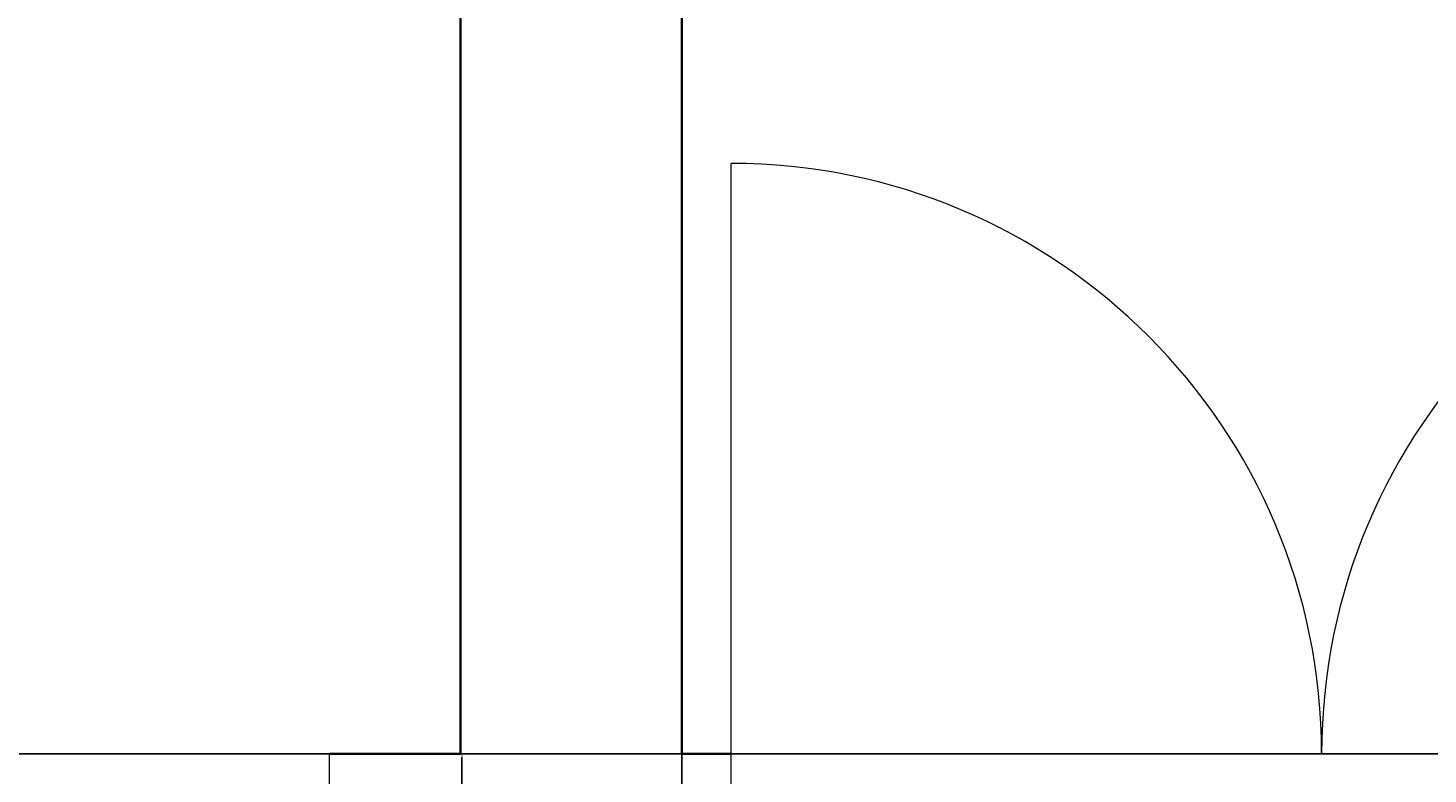
# Model space of a CAD drawing. Units: feet. Extents: x 1654 to 2985, y 1348 to 2230.
# Tile 32 of 53: x 2044 to 2100, y 1750 to 1781. Entities that reach past the tile are written whole.
import ezdxf

# ---------------------------------------------------------------- set-up
doc = ezdxf.new("R2010")
doc.units = ezdxf.units.FT
for name, color, linetype, lineweight in [('A-ANNO-DIMS', 2, 'Continuous', 18), ('A-DOOR', 3, 'Continuous', 18), ('A-WALL', 7, 'Continuous', 35), ('A-WALL-OPEN', 4, 'Continuous', 18)]:
    doc.layers.add(name, color=color, linetype=linetype, lineweight=lineweight)
doc.styles.get("Standard").update_dxf_attribs({"font": 'arial.ttf'})
doc.dimstyles.get("Standard").update_dxf_attribs({"dimtxt": 0.18, "dimasz": 0.18, "dimexe": 0.18, "dimexo": 0.0625, "dimgap": 0.09, "dimtad": 0, "dimtih": 1, "dimtoh": 1, "dimdec": 4, "dimzin": 0, "dimdsep": 46, "dimtxsty": 'Standard', "dimcen": 0.09, "dimadec": 0, "dimazin": 0, "dimtfac": 1, "dimtdec": 4, "dimtofl": 0, "dimtmove": 0, "dimatfit": 3, "dimfxl": 1, "dimtolj": 1, "dimtzin": 0, "dimarcsym": 0})

# ---------------------------------------------------------------- blocks, each defined once
blk = doc.blocks.new('DOOR-ENTRY-PAIR')
for p, q in [((0, -9), (0, 24)), ((48, -9), (48, 24))]:
    blk.add_line(p, q)
for centre, start, end in [((0, 0), 0, 90), ((48, 0), 90, 180)]:
    blk.add_arc(centre, 24, start, end)
blk = doc.blocks.new('OPENING-PUJA')
for p, q in [((0, 9), (0, 0)), ((36, 9), (36, 0)), ((0, 4.5), (36, 4.5))]:
    blk.add_line(p, q)
blk = doc.blocks.new('*D69')
at = {"layer": 'A-ANNO-DIMS', "color": 0, "lineweight": -2, "transparency": 16777216}
for p, q in [((2055.819, 1751.255), (2061.337, 1751.255)), ((2061.157, 1751.075), (2061.157, 1746.937)), ((2061.157, 1742.435), (2061.157, 1746.573)), ((2055.819, 1742.255), (2061.337, 1742.255))]:
    blk.add_line(p, q, dxfattribs=at)
at = {"layer": 'A-ANNO-DIMS', "color": 0, "transparency": 16777216}
for points in [[(2061.127, 1751.075), (2061.187, 1751.075), (2061.157, 1751.255)], [(2061.127, 1742.435), (2061.187, 1742.435), (2061.157, 1742.255)]]:
    blk.add_solid(points, dxfattribs=at)
at = {"layer": 'Defpoints', "color": 0, "transparency": 16777216}
for p in [(2055.757, 1751.255), (2061.157, 1751.255), (2055.757, 1742.255)]:
    blk.add_point(p, dxfattribs=at)
at = {"layer": 'A-ANNO-DIMS', "color": 0, "transparency": 16777216, "insert": (2061.157, 1746.755), "char_height": 0.18, "attachment_point": 5}
blk.add_mtext('\\A1;9 TYP.', dxfattribs=at)
blk = doc.blocks.new('*D80')
at = {"layer": 'A-ANNO-DIMS', "color": 0, "lineweight": -2, "transparency": 16777216}
for p, q in [((2070.092, 2039.192), (2070.092, 1534.075)), ((2202.092, 2039.192), (2202.092, 1534.075)), ((2070.272, 1534.255), (2135.813, 1534.255)), ((2201.912, 1534.255), (2136.372, 1534.255))]:
    blk.add_line(p, q, dxfattribs=at)
at = {"layer": 'A-ANNO-DIMS', "color": 0, "transparency": 16777216}
for points in [[(2070.272, 1534.285), (2070.272, 1534.225), (2070.092, 1534.255)], [(2201.912, 1534.285), (2201.912, 1534.225), (2202.092, 1534.255)]]:
    blk.add_solid(points, dxfattribs=at)
at = {"layer": 'Defpoints', "color": 0, "transparency": 16777216}
for p in [(2070.092, 2039.255), (2202.092, 2039.255), (2202.092, 1534.255)]:
    blk.add_point(p, dxfattribs=at)
at = {"layer": 'A-ANNO-DIMS', "color": 0, "transparency": 16777216, "insert": (2136.092, 1534.255), "char_height": 0.18, "attachment_point": 5}
blk.add_mtext('\\A1;132', dxfattribs=at)
blk = doc.blocks.new('*D91')
at = {"layer": 'A-ANNO-DIMS', "color": 0, "lineweight": -2, "transparency": 16777216}
for p, q in [((1852.155, 1801.468), (2242.272, 1801.468)), ((2242.092, 1801.288), (2242.092, 1776.544)), ((2242.092, 1751.435), (2242.092, 1776.18)), ((1852.155, 1751.255), (2242.272, 1751.255))]:
    blk.add_line(p, q, dxfattribs=at)
at = {"layer": 'A-ANNO-DIMS', "color": 0, "transparency": 16777216}
for points in [[(2242.062, 1801.288), (2242.122, 1801.288), (2242.092, 1801.468)], [(2242.062, 1751.435), (2242.122, 1751.435), (2242.092, 1751.255)]]:
    blk.add_solid(points, dxfattribs=at)
at = {"layer": 'Defpoints', "color": 0, "transparency": 16777216}
for p in [(1852.092, 1801.468), (2242.092, 1801.468), (1852.092, 1751.255)]:
    blk.add_point(p, dxfattribs=at)
at = {"layer": 'A-ANNO-DIMS', "color": 0, "transparency": 16777216, "insert": (2242.092, 1776.362), "char_height": 0.18, "attachment_point": 5}
blk.add_mtext('\\A1;50.21', dxfattribs=at)
blk = doc.blocks.new('*D98')
at = {"layer": 'A-ANNO-DIMS', "color": 0, "lineweight": -2, "transparency": 16777216}
for p, q in [((2061.03, 1811.081), (1811.912, 1811.081)), ((1812.092, 1810.901), (1812.092, 1781.35)), ((1812.092, 1751.435), (1812.092, 1780.986)), ((2061.03, 1751.255), (1811.912, 1751.255))]:
    blk.add_line(p, q, dxfattribs=at)
at = {"layer": 'A-ANNO-DIMS', "color": 0, "transparency": 16777216}
for points in [[(1812.062, 1810.901), (1812.122, 1810.901), (1812.092, 1811.081)], [(1812.062, 1751.435), (1812.122, 1751.435), (1812.092, 1751.255)]]:
    blk.add_solid(points, dxfattribs=at)
at = {"layer": 'Defpoints', "color": 0, "transparency": 16777216}
for p in [(1812.092, 1811.081), (2061.092, 1811.081), (2061.092, 1751.255)]:
    blk.add_point(p, dxfattribs=at)
at = {"layer": 'A-ANNO-DIMS', "color": 0, "transparency": 16777216, "insert": (1812.092, 1781.168), "char_height": 0.18, "attachment_point": 5}
blk.add_mtext('\\A1;59.83', dxfattribs=at)

msp = doc.modelspace()

# ---------------------------------------------------------------- linework, layer by layer
at = {"layer": 'A-WALL'}
for p, q in [((2061.0924, 1751.2549), (2061.0924, 1811.0815)), ((2070.0924, 1751.2549), (2070.0924, 1811.0815)), ((2061.0924, 1751.2549), (2055.7567, 1751.2549)), ((2072.0924, 1751.2549), (2070.0924, 1751.2549))]:
    msp.add_line(p, q, dxfattribs=at)

# ---------------------------------------------------------------- block references
at = {"layer": 'A-DOOR'}
msp.add_blockref('DOOR-ENTRY-PAIR', (2072.0924, 1751.2549), dxfattribs=at)
at = {"layer": 'A-WALL-OPEN'}
msp.add_blockref('OPENING-PUJA', (2019.757, 1742.255), dxfattribs=at)

# ---------------------------------------------------------------- dimensions: what is measured, and where the dimension line sits
at = {"layer": 'A-ANNO-DIMS'}
dim = msp.add_linear_dim(base=(2202.0924, 1534.2549), p1=(2070.0924, 2039.2549), p2=(2202.0924, 2039.2549), dimstyle='Standard', override={"dimdec": 0, "dimlfac": 1, "dimrnd": 0, "dimzin": 0, "dimdsep": 46, "dimlunit": 2}, dxfattribs=at)
dim.commit()
dim.dimension.update_dxf_attribs({"geometry": '*D80', "text_midpoint": (2136.0924, 1534.2549)})
for base, p1, p2, picture, middle in [((1812.0924, 1811.0815), (2061.0924, 1751.2549), (2061.0924, 1811.0815), '*D98', (1812.0924, 1781.1682)), ((2242.0924, 1801.4683), (1852.0924, 1751.2549), (1852.0924, 1801.4683), '*D91', (2242.0924, 1776.3616))]:
    dim = msp.add_linear_dim(base=base, p1=p1, p2=p2, angle=90, dimstyle='Standard', override={"dimdec": 2, "dimlfac": 1, "dimrnd": 0, "dimzin": 0, "dimdsep": 46, "dimlunit": 2}, dxfattribs=at)
    dim.commit()
    dim.dimension.update_dxf_attribs({"geometry": picture, "text_midpoint": middle})
dim = msp.add_linear_dim(base=(2061.1567, 1751.2549), p1=(2055.7567, 1742.2549), p2=(2055.7567, 1751.2549), angle=90, text='<> TYP.', dimstyle='Standard', override={"dimdec": 0, "dimlfac": 1, "dimrnd": 0, "dimzin": 0, "dimdsep": 46, "dimlunit": 2}, dxfattribs=at)
dim.commit()
dim.dimension.update_dxf_attribs({"geometry": '*D69', "text_midpoint": (2061.1567, 1746.7549)})

doc.saveas('drawing.dxf')
